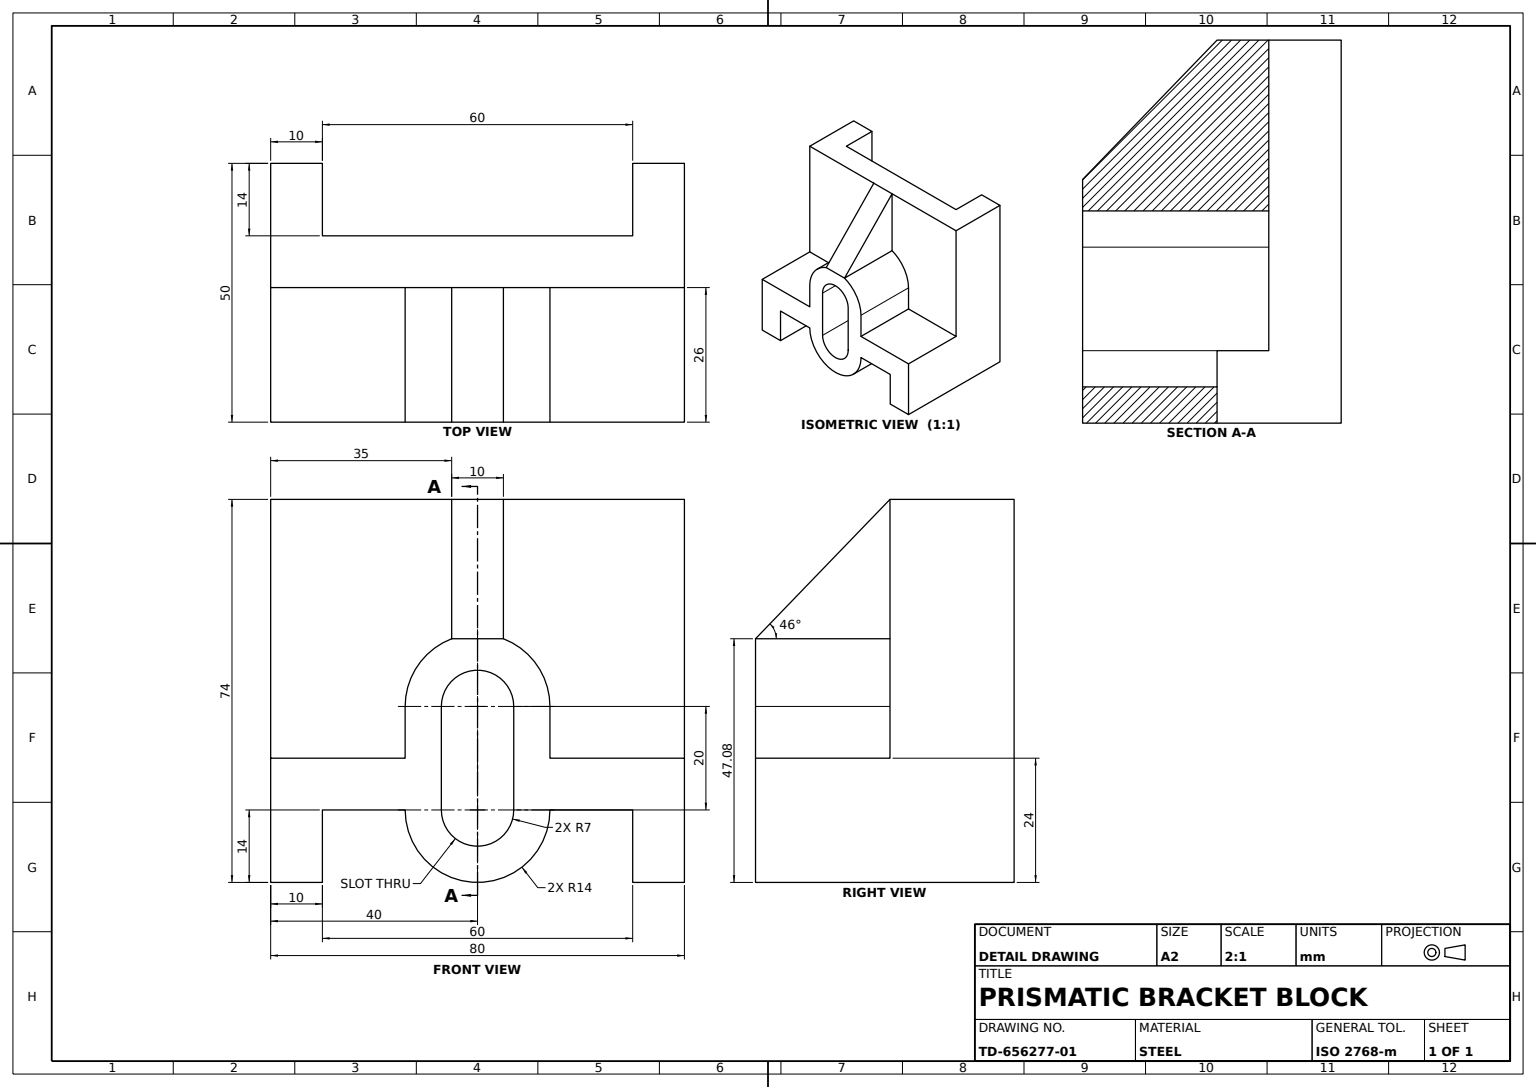
from build123d import *

# Parameters (mm, degrees)
BASE_BODY_DEPTH       = 50
BACK_WALL_SKETCH_W    = 80
BACK_WALL_SKETCH_H    = 24
BACK_WALL_DEPTH       = 50
WALL_NOTCH_SKETCH_W   = 60
WALL_NOTCH_SKETCH_H   = 14
WALL_NOTCH_CUT_DEPTH  = 120.899958299
SLOT_BOSS_DEPTH       = 26
SLOT_CUT_14MM_DEPTH   = 107.77078252
RIB_SKETCH_W          = 10
RIB_SKETCH_H          = 27
REINFORCING_RIB_DEPTH = 26
TRIM_CUT_DEPTH        = 84.815273071
TRIM_CUT_DEPTH_BACK   = 26


with BuildPart() as part:
    # Base Profile Sketch → Base Body (new body)
    with BuildSketch(Plane.XY):
        Polygon((0, 0), (40, 0), (80, 0), (80, -24), (70, -24), (70, -10), (10, -10), (10, -24), (0, -24), align=None)
    extrude(amount=-BASE_BODY_DEPTH)

    # Back Wall Sketch → Back Wall (add)
    with BuildSketch(Plane(origin=(0, 0, 0), x_dir=(1, 0, 0), z_dir=(0, 1, 0))):
        with Locations((40, 38)):
            Rectangle(BACK_WALL_SKETCH_W, BACK_WALL_SKETCH_H)
    extrude(amount=BACK_WALL_DEPTH)

    # Wall Notch Sketch → Wall Notch Cut (cut, through all)
    with BuildSketch(Plane(origin=(0, 50, 0), x_dir=(1, 0, 0), z_dir=(0, 1, 0))):
        with Locations((40, 43)):
            Rectangle(WALL_NOTCH_SKETCH_W, WALL_NOTCH_SKETCH_H)
    extrude(amount=-WALL_NOTCH_CUT_DEPTH, mode=Mode.SUBTRACT)

    # Slot Boss Sketch → Slot Boss (add)
    with BuildSketch(Plane.XY):
        with BuildLine():
            Line((26, 10), (26, -10))
            ThreePointArc((26, -10), (40, -24), (54, -10))
            Line((54, -10), (54, 10))
            ThreePointArc((54, 10), (40, 24), (26, 10))
        make_face()
    extrude(amount=-SLOT_BOSS_DEPTH)

    # Slot Sketch → Slot Cut 14mm (cut, through all)
    with BuildSketch(Plane.XY):
        with BuildLine():
            Line((33, -10), (33, 10))
            ThreePointArc((33, 10), (40, 17), (47, 10))
            Line((47, 10), (47, -10))
            ThreePointArc((47, -10), (40, -17), (33, -10))
        make_face()
    extrude(amount=-SLOT_CUT_14MM_DEPTH, mode=Mode.SUBTRACT)

    # Rib Sketch → Reinforcing Rib (add)
    with BuildSketch(Plane.XY.offset(-26)):
        with Locations((40, 36.5)):
            Rectangle(RIB_SKETCH_W, RIB_SKETCH_H)
    extrude(amount=REINFORCING_RIB_DEPTH)

    # Trim Line Sketch → Trim Cut (cut, two sides: drawn at the far end of the back side and taken through both)
    with BuildSketch(Plane.ZY.offset(-35).offset(-TRIM_CUT_DEPTH_BACK)):
        Polygon((-141.918286791, 170.034737621), (-26, 50), (0, 23.076696831), (115.918286791, -96.95804079), (355.987762032, 134.878532791), (98.151188451, 401.871311202), align=None)
    extrude(amount=TRIM_CUT_DEPTH + TRIM_CUT_DEPTH_BACK, mode=Mode.SUBTRACT)


solid = part.part
